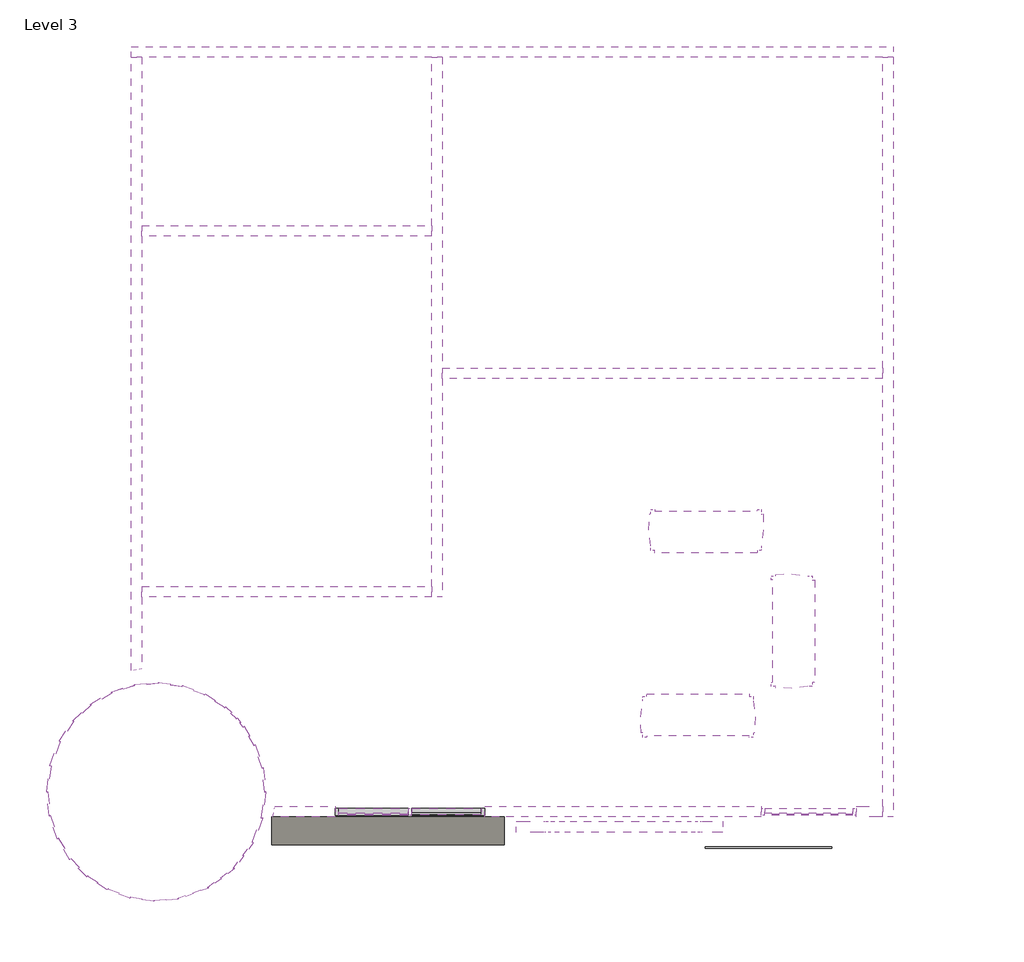
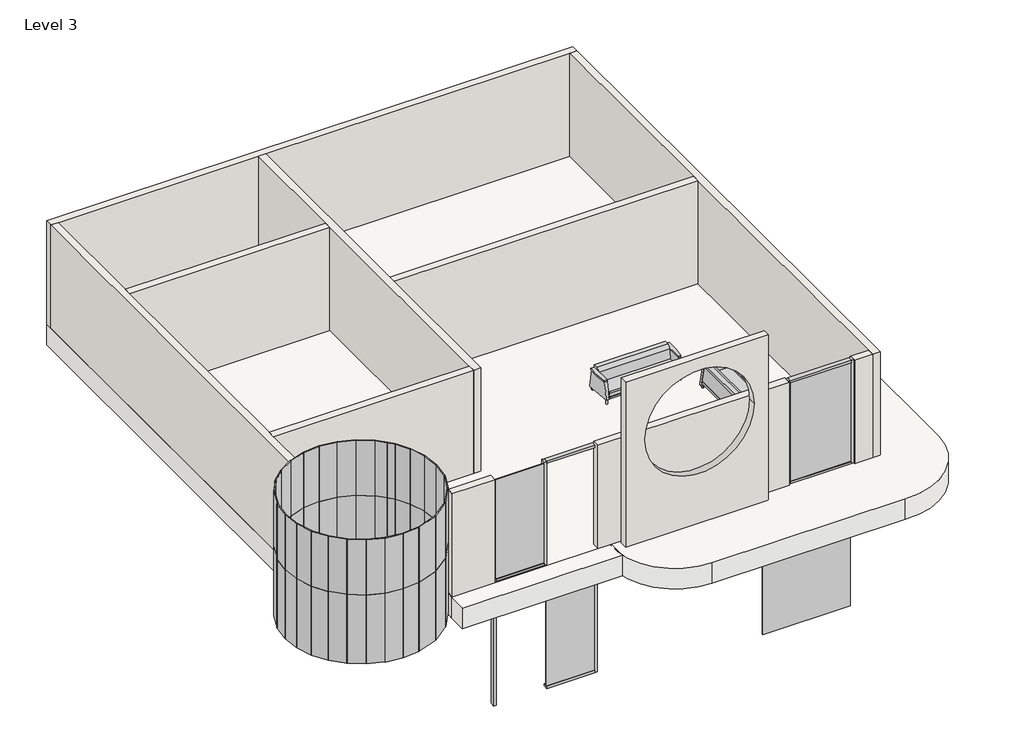
# One storey, incomplete: 60 plates, 11 members, 11 walls, 3 furniture elements, 2 slabs.
"""IFC4 building model written with IfcOpenShell, lengths in millimetres."""

from ifc_helpers import new_model, si_unit, point, frame, frame_2d, origin, place, context, project, spatial, polyline, circle_curve, trimmed, segment, composite_curve, outline, extrude, faceted_brep, transform, mapped, element, save
from ifc_brep_helpers import plane_surface, revolved_surface, advanced_brep
from components import furniture_aff9b2fb, member_eaba9652, member_3f395ae9, member_0c868e12, member_7bc42366, system_panel_glazed_f1c144f9, system_panel_glazed_8ed2b2ee, system_panel_glazed_c7815b78, system_panel_glazed_220ba5f3, system_panel_glazed_11fb153e, system_panel_glazed_2f540b85, system_panel_glazed_4848e608, system_panel_glazed_8b35a0ff, system_panel_glazed_87282c25, system_panel_glazed_6d1bb68c, system_panel_glazed_cb3ffd69, system_panel_glazed_404d015f, system_panel_glazed_7b556abe, system_panel_glazed_c60cfc80, system_panel_glazed_370bf902

model = new_model("IFC4")

# Units and contexts
model_context = context("Model", 3, world=origin())
ifc_project = project(units=[si_unit("LENGTHUNIT", "METRE", prefix="MILLI")], contexts=[model_context])

# Site, building, storey
site = spatial("IfcSite", under=ifc_project)
building = spatial("IfcBuilding", under=site)
storey = spatial("IfcBuildingStorey", under=building, Name="Level 3", Elevation=6096.0)

# Furniture
placement = place(None, origin())
furniture_shape = furniture_aff9b2fb(model_context)
element("IfcFurniture", 1, ObjectType="Sofa-Pensi : 84\"", at=placement, inside=storey, context=model_context, shape_type="MappedRepresentation", body=[
    mapped(furniture_shape, transform((-2244.8524991, 3650.1964615, 7315.2), x_axis=(1.0, 0.0, 0.0), y_axis=(0.0, 1.0, 0.0), z_axis=(0.0, 0.0, 1.0))),
])
element("IfcFurniture", 2, ObjectType="Sofa-Pensi : 84\"", at=placement, inside=storey, context=model_context, shape_type="MappedRepresentation", body=[
    mapped(furniture_shape, transform((-12.736413, 1720.492712, 7315.2), x_axis=(0.0, 1.0, 0.0), y_axis=(-1.0, 0.0, 0.0), z_axis=(0.0, 0.0, 1.0))),
])
element("IfcFurniture", 3, ObjectType="Sofa-Pensi : 84\"", at=placement, inside=storey, context=model_context, shape_type="MappedRepresentation", body=[
    mapped(furniture_shape, transform((-1840.0399991, 648.4161336, 7315.2), x_axis=(-1.0, 0.0, 0.0), y_axis=(0.0, -1.0, 0.0), z_axis=(0.0, 0.0, 1.0))),
])

# Members
member_shape = member_eaba9652(model_context)
element("IfcMember", 4, ObjectType="Rectangular Mullion : 2.5\" x 5\" rectangular", at=placement, inside=storey, context=model_context, shape_type="MappedRepresentation", body=[
    mapped(member_shape, transform((-7672.5789001, -1482.8937024, 7315.2), x_axis=(-1.0, 0.0, 0.0), y_axis=(0.0, 1.0, 0.0), z_axis=(0.0, 0.0, -1.0))),
])
member_2_shape = member_3f395ae9(model_context)
element("IfcMember", 5, ObjectType="Rectangular Mullion : 2.5\" x 5\" rectangular", at=placement, inside=storey, context=model_context, shape_type="MappedRepresentation", body=[
    mapped(member_2_shape, transform((-9111.7115512, -1482.8937024, 3657.6), x_axis=(-1.0, 0.0, 0.0), y_axis=(0.0, 1.0, 0.0), z_axis=(0.0, 0.0, -1.0))),
])
element("IfcMember", 6, ObjectType="Rectangular Mullion : 2.5\" x 5\" rectangular", at=placement, inside=storey, context=model_context, shape_type="MappedRepresentation", body=[
    mapped(member_2_shape, transform((-899.4462491, -1482.8937024, 7315.2), x_axis=(-1.0, 0.0, 0.0), y_axis=(0.0, 1.0, 0.0), z_axis=(0.0, 0.0, -1.0))),
])
element("IfcMember", 7, ObjectType="Rectangular Mullion : 2.5\" x 5\" rectangular", at=placement, inside=storey, context=model_context, shape_type="MappedRepresentation", body=[
    mapped(member_2_shape, transform((-6233.4462491, -1482.8937024, 6705.6), x_axis=(1.0, 0.0, 0.0), y_axis=(0.0, 1.0, 0.0), z_axis=(0.0, 0.0, 1.0))),
])
element("IfcMember", 8, ObjectType="Rectangular Mullion : 2.5\" x 5\" rectangular", at=placement, inside=storey, context=model_context, shape_type="MappedRepresentation", body=[
    mapped(member_2_shape, transform((929.3537509, -1482.8937024, 10363.2), x_axis=(1.0, 0.0, 0.0), y_axis=(0.0, 1.0, 0.0), z_axis=(0.0, 0.0, 1.0))),
])
member_3_shape = member_0c868e12(model_context)
element("IfcMember", 9, ObjectType="Rectangular Mullion : 2.5\" x 5\" rectangular", at=placement, inside=storey, context=model_context, shape_type="MappedRepresentation", body=[
    mapped(member_3_shape, transform((-9048.2115512, -1482.8937024, 6705.6), x_axis=(0.0, 0.0, 1.0), y_axis=(0.0, 1.0, 0.0), z_axis=(-1.0, 0.0, 0.0))),
])
element("IfcMember", 10, ObjectType="Rectangular Mullion : 2.5\" x 5\" rectangular", at=placement, inside=storey, context=model_context, shape_type="MappedRepresentation", body=[
    mapped(member_3_shape, transform((-7640.8289001, -1482.8937024, 10363.2), x_axis=(0.0, 0.0, 1.0), y_axis=(0.0, 1.0, 0.0), z_axis=(-1.0, 0.0, 0.0))),
])
element("IfcMember", 11, ObjectType="Rectangular Mullion : 2.5\" x 5\" rectangular", at=placement, inside=storey, context=model_context, shape_type="MappedRepresentation", body=[
    mapped(member_3_shape, transform((-6296.9462491, -1482.8937024, 3657.6), x_axis=(0.0, 0.0, -1.0), y_axis=(0.0, 1.0, 0.0), z_axis=(1.0, 0.0, 0.0))),
])
element("IfcMember", 12, ObjectType="Rectangular Mullion : 2.5\" x 5\" rectangular", at=placement, inside=storey, context=model_context, shape_type="MappedRepresentation", body=[
    mapped(member_3_shape, transform((-7704.3289001, -1482.8937024, 7315.2), x_axis=(0.0, 0.0, -1.0), y_axis=(0.0, 1.0, 0.0), z_axis=(1.0, 0.0, 0.0))),
])
member_4_shape = member_7bc42366(model_context)
element("IfcMember", 13, ObjectType="Rectangular Mullion : 2.5\" x 5\" rectangular", at=placement, inside=storey, context=model_context, shape_type="MappedRepresentation", body=[
    mapped(member_4_shape, transform((-835.9462491, -1482.8937024, 10363.2), x_axis=(0.0, 0.0, 1.0), y_axis=(0.0, 1.0, 0.0), z_axis=(-1.0, 0.0, 0.0))),
])
element("IfcMember", 14, ObjectType="Rectangular Mullion : 2.5\" x 5\" rectangular", at=placement, inside=storey, context=model_context, shape_type="MappedRepresentation", body=[
    mapped(member_4_shape, transform((865.8537509, -1482.8937024, 7315.2), x_axis=(0.0, 0.0, -1.0), y_axis=(0.0, 1.0, 0.0), z_axis=(1.0, 0.0, 0.0))),
])

# Plates
system_panel_glazed_shape = system_panel_glazed_f1c144f9(model_context)
element("IfcPlate", 15, ObjectType="System Panel : Glazed", at=placement, inside=storey, context=model_context, shape_type="MappedRepresentation", body=[
    mapped(system_panel_glazed_shape, transform((-14541.9245022, -346.5978939, 7315.2), x_axis=(-0.3551689475306269, -0.9348021281051873, 0.0), y_axis=(0.9348021281051873, -0.3551689475306269, 0.0), z_axis=(0.0, 0.0, 1.0))),
])
element("IfcPlate", 16, ObjectType="System Panel : Glazed", at=placement, inside=storey, context=model_context, shape_type="MappedRepresentation", body=[
    mapped(system_panel_glazed_shape, transform((-10582.1178502, -1851.0877948, 7315.2), x_axis=(0.35516894753064066, 0.934802128105182, 0.0), y_axis=(-0.934802128105182, 0.35516894753064066, 0.0), z_axis=(0.0, 0.0, 1.0))),
])
element("IfcPlate", 17, ObjectType="System Panel : Glazed", at=placement, inside=storey, context=model_context, shape_type="MappedRepresentation", body=[
    mapped(system_panel_glazed_shape, transform((-10459.5232171, -1354.5613954, 7315.2), x_axis=(0.12073632210407238, 0.9926846128175765, 0.0), y_axis=(-0.9926846128175765, 0.12073632210407238, 0.0), z_axis=(0.0, 0.0, 1.0))),
])
element("IfcPlate", 18, ObjectType="System Panel : Glazed", at=placement, inside=storey, context=model_context, shape_type="MappedRepresentation", body=[
    mapped(system_panel_glazed_shape, transform((-14664.5191354, -843.1242933, 7315.2), x_axis=(-0.12073632210406242, -0.9926846128175777, 0.0), y_axis=(0.9926846128175777, -0.12073632210406242, 0.0), z_axis=(0.0, 0.0, 1.0))),
])
system_panel_glazed_2_shape = system_panel_glazed_8ed2b2ee(model_context)
element("IfcPlate", 19, ObjectType="System Panel : Glazed", at=placement, inside=storey, context=model_context, shape_type="MappedRepresentation", body=[
    mapped(system_panel_glazed_2_shape, transform((-11841.3777431, -3082.3793017, 7315.2), x_axis=(0.9398911711666007, 0.34147413718036645, 0.0), y_axis=(-0.34147413718036645, 0.9398911711666007, 0.0), z_axis=(0.0, 0.0, 1.0))),
])
element("IfcPlate", 20, ObjectType="System Panel : Glazed", at=placement, inside=storey, context=model_context, shape_type="MappedRepresentation", body=[
    mapped(system_panel_glazed_2_shape, transform((-10858.9635423, -2345.1728692, 7315.2), x_axis=(0.5905687200141164, 0.8069873524045393, 0.0), y_axis=(-0.8069873524045393, 0.5905687200141164, 0.0), z_axis=(0.0, 0.0, 1.0))),
])
element("IfcPlate", 21, ObjectType="System Panel : Glazed", at=placement, inside=storey, context=model_context, shape_type="MappedRepresentation", body=[
    mapped(system_panel_glazed_2_shape, transform((-11295.3522982, -2786.8279712, 7315.2), x_axis=(0.7998453025525061, 0.6002062078858317, 0.0), y_axis=(-0.6002062078858317, 0.7998453025525061, 0.0), z_axis=(0.0, 0.0, 1.0))),
])
system_panel_glazed_3_shape = system_panel_glazed_c7815b78(model_context)
element("IfcPlate", 22, ObjectType="System Panel : Glazed", at=placement, inside=storey, context=model_context, shape_type="MappedRepresentation", body=[
    mapped(system_panel_glazed_3_shape, transform((-10454.4737362, -864.5204039, 7315.2), x_axis=(-0.11050163420416613, 0.993875942378227, 0.0), y_axis=(-0.993875942378227, -0.11050163420416613, 0.0), z_axis=(0.0, 0.0, 1.0))),
])
element("IfcPlate", 23, ObjectType="System Panel : Glazed", at=placement, inside=storey, context=model_context, shape_type="MappedRepresentation", body=[
    mapped(system_panel_glazed_3_shape, transform((-14669.5686163, -1333.1652848, 7315.2), x_axis=(0.11050163420415138, -0.9938759423782286, 0.0), y_axis=(0.9938759423782286, 0.11050163420415138, 0.0), z_axis=(0.0, 0.0, 1.0))),
])
element("IfcPlate", 24, ObjectType="System Panel : Glazed", at=placement, inside=storey, context=model_context, shape_type="MappedRepresentation", body=[
    mapped(system_panel_glazed_3_shape, transform((-11410.1424167, 681.5611944, 7315.2), x_axis=(-0.8396018558176894, 0.5432022861766066, 0.0), y_axis=(-0.5432022861766066, -0.8396018558176894, 0.0), z_axis=(0.0, 0.0, 1.0))),
])
element("IfcPlate", 25, ObjectType="System Panel : Glazed", at=placement, inside=storey, context=model_context, shape_type="MappedRepresentation", body=[
    mapped(system_panel_glazed_3_shape, transform((-13212.0893695, 919.590846, 7315.2), x_axis=(-0.9518517343814786, -0.3065587639506839, 0.0), y_axis=(0.3065587639506839, -0.9518517343814786, 0.0), z_axis=(0.0, 0.0, 1.0))),
])
element("IfcPlate", 26, ObjectType="System Panel : Glazed", at=placement, inside=storey, context=model_context, shape_type="MappedRepresentation", body=[
    mapped(system_panel_glazed_3_shape, transform((-12839.7224363, -3201.1142893, 7315.2), x_axis=(0.9913878918151698, -0.1309581916577702, 0.0), y_axis=(0.1309581916577702, 0.9913878918151698, 0.0), z_axis=(0.0, 0.0, 1.0))),
])
element("IfcPlate", 27, ObjectType="System Panel : Glazed", at=placement, inside=storey, context=model_context, shape_type="MappedRepresentation", body=[
    mapped(system_panel_glazed_3_shape, transform((-14365.783041, -2213.7896382, 7315.2), x_axis=(0.5257859322352114, -0.8506169252157811, 0.0), y_axis=(0.8506169252157811, 0.5257859322352114, 0.0), z_axis=(0.0, 0.0, 1.0))),
])
element("IfcPlate", 28, ObjectType="System Panel : Glazed", at=placement, inside=storey, context=model_context, shape_type="MappedRepresentation", body=[
    mapped(system_panel_glazed_3_shape, transform((-13713.8999358, -2879.2468831, 7315.2), x_axis=(0.8396018558176805, -0.5432022861766201, 0.0), y_axis=(0.5432022861766201, 0.8396018558176805, 0.0), z_axis=(0.0, 0.0, 1.0))),
])
element("IfcPlate", 29, ObjectType="System Panel : Glazed", at=placement, inside=storey, context=model_context, shape_type="MappedRepresentation", body=[
    mapped(system_panel_glazed_3_shape, transform((-14014.4059364, 446.2272921, 7315.2), x_axis=(-0.7286232370002992, -0.6849147235263715, 0.0), y_axis=(0.6849147235263715, -0.7286232370002992, 0.0), z_axis=(0.0, 0.0, 1.0))),
])
element("IfcPlate", 30, ObjectType="System Panel : Glazed", at=placement, inside=storey, context=model_context, shape_type="MappedRepresentation", body=[
    mapped(system_panel_glazed_3_shape, transform((-12284.3199161, 1003.4286006, 7315.2), x_axis=(-0.9913878918151723, 0.1309581916577514, 0.0), y_axis=(-0.1309581916577514, -0.9913878918151723, 0.0), z_axis=(0.0, 0.0, 1.0))),
])
element("IfcPlate", 31, ObjectType="System Panel : Glazed", at=placement, inside=storey, context=model_context, shape_type="MappedRepresentation", body=[
    mapped(system_panel_glazed_3_shape, transform((-12752.8652893, 1013.0855973, 7315.2), x_axis=(-0.9959419324521102, -0.08999815100076568, 0.0), y_axis=(0.08999815100076568, -0.9959419324521102, 0.0), z_axis=(0.0, 0.0, 1.0))),
])
element("IfcPlate", 32, ObjectType="System Panel : Glazed", at=placement, inside=storey, context=model_context, shape_type="MappedRepresentation", body=[
    mapped(system_panel_glazed_3_shape, transform((-11829.3381514, 891.0915272, 7315.2), x_axis=(-0.9384120429483949, 0.34551821608913763, 0.0), y_axis=(-0.34551821608913763, -0.9384120429483949, 0.0), z_axis=(0.0, 0.0, 1.0))),
])
element("IfcPlate", 33, ObjectType="System Panel : Glazed", at=placement, inside=storey, context=model_context, shape_type="MappedRepresentation", body=[
    mapped(system_panel_glazed_3_shape, transform((-10557.4115054, -407.3204039, 7315.2), x_axis=(-0.3261077326604367, 0.9453326116764772, 0.0), y_axis=(-0.9453326116764772, -0.3261077326604367, 0.0), z_axis=(0.0, 0.0, 1.0))),
])
element("IfcPlate", 34, ObjectType="System Panel : Glazed", at=placement, inside=storey, context=model_context, shape_type="MappedRepresentation", body=[
    mapped(system_panel_glazed_3_shape, transform((-12371.1770631, -3210.771286, 7315.2), x_axis=(0.9959419324521115, 0.08999815100075, 0.0), y_axis=(-0.08999815100075, 0.9959419324521115, 0.0), z_axis=(0.0, 0.0, 1.0))),
])
element("IfcPlate", 35, ObjectType="System Panel : Glazed", at=placement, inside=storey, context=model_context, shape_type="MappedRepresentation", body=[
    mapped(system_panel_glazed_3_shape, transform((-13294.7042011, -3088.7772159, 7315.2), x_axis=(0.9384120429483891, -0.34551821608915334, 0.0), y_axis=(0.34551821608915334, 0.9384120429483891, 0.0), z_axis=(0.0, 0.0, 1.0))),
])
element("IfcPlate", 36, ObjectType="System Panel : Glazed", at=placement, inside=storey, context=model_context, shape_type="MappedRepresentation", body=[
    mapped(system_panel_glazed_3_shape, transform((-14076.8350959, -2582.7572647, 7315.2), x_axis=(0.6997834615185511, -0.7143550286692988, 0.0), y_axis=(0.7143550286692988, 0.6997834615185511, 0.0), z_axis=(0.0, 0.0, 1.0))),
])
element("IfcPlate", 37, ObjectType="System Panel : Glazed", at=placement, inside=storey, context=model_context, shape_type="MappedRepresentation", body=[
    mapped(system_panel_glazed_3_shape, transform((-14566.6308471, -1790.3652848, 7315.2), x_axis=(0.32610773266042153, -0.9453326116764824, 0.0), y_axis=(0.9453326116764824, 0.32610773266042153, 0.0), z_axis=(0.0, 0.0, 1.0))),
])
element("IfcPlate", 38, ObjectType="System Panel : Glazed", at=placement, inside=storey, context=model_context, shape_type="MappedRepresentation", body=[
    mapped(system_panel_glazed_3_shape, transform((-14318.3113206, 89.4787227, 7315.2), x_axis=(-0.5603879632167612, -0.8282302401396425, 0.0), y_axis=(0.8282302401396425, -0.5603879632167612, 0.0), z_axis=(0.0, 0.0, 1.0))),
])
element("IfcPlate", 39, ObjectType="System Panel : Glazed", at=placement, inside=storey, context=model_context, shape_type="MappedRepresentation", body=[
    mapped(system_panel_glazed_3_shape, transform((-13639.5625299, 727.5108588, 7315.2), x_axis=(-0.8612707706620223, -0.508146297441245, 0.0), y_axis=(0.508146297441245, -0.8612707706620223, 0.0), z_axis=(0.0, 0.0, 1.0))),
])
system_panel_glazed_4_shape = system_panel_glazed_220ba5f3(model_context)
element("IfcPlate", 40, ObjectType="System Panel : Glazed", at=placement, inside=storey, context=model_context, shape_type="MappedRepresentation", body=[
    mapped(system_panel_glazed_4_shape, transform((-10742.3305673, -4.7597883, 7315.2), x_axis=(-0.5152811917631037, 0.8570211744263939, 0.0), y_axis=(-0.8570211744263939, -0.5152811917631037, 0.0), z_axis=(0.0, 0.0, 1.0))),
])
system_panel_glazed_5_shape = system_panel_glazed_11fb153e(model_context)
element("IfcPlate", 41, ObjectType="System Panel : Glazed", at=placement, inside=storey, context=model_context, shape_type="MappedRepresentation", body=[
    mapped(system_panel_glazed_5_shape, transform((-11098.0043985, 445.2241463, 7315.2), x_axis=(-0.7256671855033587, 0.6880458821064435, 0.0), y_axis=(-0.6880458821064435, -0.7256671855033587, 0.0), z_axis=(0.0, 0.0, 1.0))),
])
system_panel_glazed_6_shape = system_panel_glazed_2f540b85(model_context)
element("IfcPlate", 42, ObjectType="System Panel : Glazed", at=placement, inside=storey, context=model_context, shape_type="MappedRepresentation", body=[
    mapped(system_panel_glazed_6_shape, transform((-10917.0903061, 255.9395759, 7315.2), x_axis=(-0.6357445726375757, 0.7718995001694627, 0.0), y_axis=(-0.7718995001694627, -0.6357445726375757, 0.0), z_axis=(0.0, 0.0, 1.0))),
])
system_panel_glazed_7_shape = system_panel_glazed_4848e608(model_context)
element("IfcPlate", 43, ObjectType="System Panel : Glazed", at=placement, inside=storey, context=model_context, shape_type="MappedRepresentation", body=[
    mapped(system_panel_glazed_7_shape, transform((-14669.5686163, -1333.1652848, 9347.2), x_axis=(0.11050163420415138, -0.9938759423782286, 0.0), y_axis=(0.9938759423782286, 0.11050163420415138, 0.0), z_axis=(0.0, 0.0, 1.0))),
])
element("IfcPlate", 44, ObjectType="System Panel : Glazed", at=placement, inside=storey, context=model_context, shape_type="MappedRepresentation", body=[
    mapped(system_panel_glazed_7_shape, transform((-14365.783041, -2213.7896382, 9347.2), x_axis=(0.5257859322352114, -0.8506169252157811, 0.0), y_axis=(0.8506169252157811, 0.5257859322352114, 0.0), z_axis=(0.0, 0.0, 1.0))),
])
element("IfcPlate", 45, ObjectType="System Panel : Glazed", at=placement, inside=storey, context=model_context, shape_type="MappedRepresentation", body=[
    mapped(system_panel_glazed_7_shape, transform((-13713.8999358, -2879.2468831, 9347.2), x_axis=(0.8396018558176805, -0.5432022861766201, 0.0), y_axis=(0.5432022861766201, 0.8396018558176805, 0.0), z_axis=(0.0, 0.0, 1.0))),
])
element("IfcPlate", 46, ObjectType="System Panel : Glazed", at=placement, inside=storey, context=model_context, shape_type="MappedRepresentation", body=[
    mapped(system_panel_glazed_7_shape, transform((-12839.7224363, -3201.1142893, 9347.2), x_axis=(0.9913878918151698, -0.13095819165777017, 0.0), y_axis=(0.13095819165777017, 0.9913878918151698, 0.0), z_axis=(0.0, 0.0, 1.0))),
])
element("IfcPlate", 47, ObjectType="System Panel : Glazed", at=placement, inside=storey, context=model_context, shape_type="MappedRepresentation", body=[
    mapped(system_panel_glazed_7_shape, transform((-12371.1770631, -3210.771286, 9347.2), x_axis=(0.9959419324521115, 0.08999815100075002, 0.0), y_axis=(-0.08999815100075002, 0.9959419324521115, 0.0), z_axis=(0.0, 0.0, 1.0))),
])
element("IfcPlate", 48, ObjectType="System Panel : Glazed", at=placement, inside=storey, context=model_context, shape_type="MappedRepresentation", body=[
    mapped(system_panel_glazed_7_shape, transform((-13294.7042011, -3088.7772159, 9347.2), x_axis=(0.9384120429483891, -0.34551821608915334, 0.0), y_axis=(0.34551821608915334, 0.9384120429483891, 0.0), z_axis=(0.0, 0.0, 1.0))),
])
element("IfcPlate", 49, ObjectType="System Panel : Glazed", at=placement, inside=storey, context=model_context, shape_type="MappedRepresentation", body=[
    mapped(system_panel_glazed_7_shape, transform((-14076.8350959, -2582.7572647, 9347.2), x_axis=(0.6997834615185511, -0.7143550286692988, 0.0), y_axis=(0.7143550286692988, 0.6997834615185511, 0.0), z_axis=(0.0, 0.0, 1.0))),
])
element("IfcPlate", 50, ObjectType="System Panel : Glazed", at=placement, inside=storey, context=model_context, shape_type="MappedRepresentation", body=[
    mapped(system_panel_glazed_7_shape, transform((-14566.6308471, -1790.3652848, 9347.2), x_axis=(0.32610773266042153, -0.9453326116764824, 0.0), y_axis=(0.9453326116764824, 0.32610773266042153, 0.0), z_axis=(0.0, 0.0, 1.0))),
])
element("IfcPlate", 51, ObjectType="System Panel : Glazed", at=placement, inside=storey, context=model_context, shape_type="MappedRepresentation", body=[
    mapped(system_panel_glazed_7_shape, transform((-10454.4737362, -864.5204039, 9347.2), x_axis=(-0.11050163420416614, 0.993875942378227, 0.0), y_axis=(-0.993875942378227, -0.11050163420416614, 0.0), z_axis=(0.0, 0.0, 1.0))),
])
element("IfcPlate", 52, ObjectType="System Panel : Glazed", at=placement, inside=storey, context=model_context, shape_type="MappedRepresentation", body=[
    mapped(system_panel_glazed_7_shape, transform((-10557.4115054, -407.3204039, 9347.2), x_axis=(-0.32610773266043674, 0.9453326116764772, 0.0), y_axis=(-0.9453326116764772, -0.32610773266043674, 0.0), z_axis=(0.0, 0.0, 1.0))),
])
element("IfcPlate", 53, ObjectType="System Panel : Glazed", at=placement, inside=storey, context=model_context, shape_type="MappedRepresentation", body=[
    mapped(system_panel_glazed_7_shape, transform((-11410.1424167, 681.5611944, 9347.2), x_axis=(-0.8396018558176894, 0.5432022861766066, 0.0), y_axis=(-0.5432022861766066, -0.8396018558176894, 0.0), z_axis=(0.0, 0.0, 1.0))),
])
element("IfcPlate", 54, ObjectType="System Panel : Glazed", at=placement, inside=storey, context=model_context, shape_type="MappedRepresentation", body=[
    mapped(system_panel_glazed_7_shape, transform((-11829.3381514, 891.0915272, 9347.2), x_axis=(-0.9384120429483949, 0.34551821608913763, 0.0), y_axis=(-0.34551821608913763, -0.9384120429483949, 0.0), z_axis=(0.0, 0.0, 1.0))),
])
element("IfcPlate", 55, ObjectType="System Panel : Glazed", at=placement, inside=storey, context=model_context, shape_type="MappedRepresentation", body=[
    mapped(system_panel_glazed_7_shape, transform((-12284.3199161, 1003.4286006, 9347.2), x_axis=(-0.9913878918151723, 0.13095819165775144, 0.0), y_axis=(-0.13095819165775144, -0.9913878918151723, 0.0), z_axis=(0.0, 0.0, 1.0))),
])
element("IfcPlate", 56, ObjectType="System Panel : Glazed", at=placement, inside=storey, context=model_context, shape_type="MappedRepresentation", body=[
    mapped(system_panel_glazed_7_shape, transform((-12752.8652893, 1013.0855973, 9347.2), x_axis=(-0.9959419324521102, -0.08999815100076569, 0.0), y_axis=(0.08999815100076569, -0.9959419324521102, 0.0), z_axis=(0.0, 0.0, 1.0))),
])
element("IfcPlate", 57, ObjectType="System Panel : Glazed", at=placement, inside=storey, context=model_context, shape_type="MappedRepresentation", body=[
    mapped(system_panel_glazed_7_shape, transform((-13212.0893695, 919.590846, 9347.2), x_axis=(-0.9518517343814786, -0.3065587639506839, 0.0), y_axis=(0.3065587639506839, -0.9518517343814786, 0.0), z_axis=(0.0, 0.0, 1.0))),
])
element("IfcPlate", 58, ObjectType="System Panel : Glazed", at=placement, inside=storey, context=model_context, shape_type="MappedRepresentation", body=[
    mapped(system_panel_glazed_7_shape, transform((-13639.5625299, 727.5108588, 9347.2), x_axis=(-0.8612707706620224, -0.5081462974412448, 0.0), y_axis=(0.5081462974412448, -0.8612707706620224, 0.0), z_axis=(0.0, 0.0, 1.0))),
])
element("IfcPlate", 59, ObjectType="System Panel : Glazed", at=placement, inside=storey, context=model_context, shape_type="MappedRepresentation", body=[
    mapped(system_panel_glazed_7_shape, transform((-14014.4059364, 446.2272921, 9347.2), x_axis=(-0.7286232370002992, -0.6849147235263715, 0.0), y_axis=(0.6849147235263715, -0.7286232370002992, 0.0), z_axis=(0.0, 0.0, 1.0))),
])
element("IfcPlate", 60, ObjectType="System Panel : Glazed", at=placement, inside=storey, context=model_context, shape_type="MappedRepresentation", body=[
    mapped(system_panel_glazed_7_shape, transform((-14318.3113206, 89.4787227, 9347.2), x_axis=(-0.5603879632167612, -0.8282302401396425, 0.0), y_axis=(0.8282302401396425, -0.5603879632167612, 0.0), z_axis=(0.0, 0.0, 1.0))),
])
system_panel_glazed_8_shape = system_panel_glazed_8b35a0ff(model_context)
element("IfcPlate", 61, ObjectType="System Panel : Glazed", at=placement, inside=storey, context=model_context, shape_type="MappedRepresentation", body=[
    mapped(system_panel_glazed_8_shape, transform((-10742.3305673, -4.7597883, 9347.2), x_axis=(-0.5152811917631037, 0.8570211744263939, 0.0), y_axis=(-0.8570211744263939, -0.5152811917631037, 0.0), z_axis=(0.0, 0.0, 1.0))),
])
system_panel_glazed_9_shape = system_panel_glazed_87282c25(model_context)
element("IfcPlate", 62, ObjectType="System Panel : Glazed", at=placement, inside=storey, context=model_context, shape_type="MappedRepresentation", body=[
    mapped(system_panel_glazed_9_shape, transform((-10917.0903061, 255.9395759, 9347.2), x_axis=(-0.6357445726375757, 0.7718995001694627, 0.0), y_axis=(-0.7718995001694627, -0.6357445726375757, 0.0), z_axis=(0.0, 0.0, 1.0))),
])
system_panel_glazed_10_shape = system_panel_glazed_6d1bb68c(model_context)
element("IfcPlate", 63, ObjectType="System Panel : Glazed", at=placement, inside=storey, context=model_context, shape_type="MappedRepresentation", body=[
    mapped(system_panel_glazed_10_shape, transform((-11098.0043985, 445.2241463, 9347.2), x_axis=(-0.7256671855033587, 0.6880458821064435, 0.0), y_axis=(-0.6880458821064435, -0.7256671855033587, 0.0), z_axis=(0.0, 0.0, 1.0))),
])
system_panel_glazed_11_shape = system_panel_glazed_cb3ffd69(model_context)
element("IfcPlate", 64, ObjectType="System Panel : Glazed", at=placement, inside=storey, context=model_context, shape_type="MappedRepresentation", body=[
    mapped(system_panel_glazed_11_shape, transform((-10582.1178502, -1851.0877948, 9347.2), x_axis=(0.3551689475306406, 0.934802128105182, 0.0), y_axis=(-0.934802128105182, 0.3551689475306406, 0.0), z_axis=(0.0, 0.0, 1.0))),
])
element("IfcPlate", 65, ObjectType="System Panel : Glazed", at=placement, inside=storey, context=model_context, shape_type="MappedRepresentation", body=[
    mapped(system_panel_glazed_11_shape, transform((-10459.5232171, -1354.5613954, 9347.2), x_axis=(0.12073632210407237, 0.9926846128175765, 0.0), y_axis=(-0.9926846128175765, 0.12073632210407237, 0.0), z_axis=(0.0, 0.0, 1.0))),
])
element("IfcPlate", 66, ObjectType="System Panel : Glazed", at=placement, inside=storey, context=model_context, shape_type="MappedRepresentation", body=[
    mapped(system_panel_glazed_11_shape, transform((-14541.9245022, -346.5978939, 9347.2), x_axis=(-0.35516894753062683, -0.9348021281051873, 0.0), y_axis=(0.9348021281051873, -0.35516894753062683, 0.0), z_axis=(0.0, 0.0, 1.0))),
])
element("IfcPlate", 67, ObjectType="System Panel : Glazed", at=placement, inside=storey, context=model_context, shape_type="MappedRepresentation", body=[
    mapped(system_panel_glazed_11_shape, transform((-14664.5191354, -843.1242933, 9347.2), x_axis=(-0.12073632210406242, -0.9926846128175777, 0.0), y_axis=(0.9926846128175777, -0.12073632210406242, 0.0), z_axis=(0.0, 0.0, 1.0))),
])
system_panel_glazed_12_shape = system_panel_glazed_404d015f(model_context)
element("IfcPlate", 68, ObjectType="System Panel : Glazed", at=placement, inside=storey, context=model_context, shape_type="MappedRepresentation", body=[
    mapped(system_panel_glazed_12_shape, transform((-11841.3777431, -3082.3793017, 9347.2), x_axis=(0.9398911711666007, 0.34147413718036645, 0.0), y_axis=(-0.34147413718036645, 0.9398911711666007, 0.0), z_axis=(0.0, 0.0, 1.0))),
])
element("IfcPlate", 69, ObjectType="System Panel : Glazed", at=placement, inside=storey, context=model_context, shape_type="MappedRepresentation", body=[
    mapped(system_panel_glazed_12_shape, transform((-10858.9635423, -2345.1728692, 9347.2), x_axis=(0.5905687200141164, 0.8069873524045393, 0.0), y_axis=(-0.8069873524045393, 0.5905687200141164, 0.0), z_axis=(0.0, 0.0, 1.0))),
])
element("IfcPlate", 70, ObjectType="System Panel : Glazed", at=placement, inside=storey, context=model_context, shape_type="MappedRepresentation", body=[
    mapped(system_panel_glazed_12_shape, transform((-11295.3522982, -2786.8279712, 9347.2), x_axis=(0.7998453025525061, 0.6002062078858317, 0.0), y_axis=(-0.6002062078858317, 0.7998453025525061, 0.0), z_axis=(0.0, 0.0, 1.0))),
])
system_panel_glazed_13_shape = system_panel_glazed_7b556abe(model_context)
element("IfcPlate", 71, ObjectType="System Panel : Glazed", at=placement, inside=storey, context=model_context, shape_type="MappedRepresentation", body=[
    mapped(system_panel_glazed_13_shape, transform((-6968.8875746, -1482.8937024, 3721.1), x_axis=(-1.0, 0.0, 0.0), y_axis=(0.0, -1.0, 0.0), z_axis=(0.0, 0.0, 1.0))),
])
element("IfcPlate", 72, ObjectType="System Panel : Glazed", at=placement, inside=storey, context=model_context, shape_type="MappedRepresentation", body=[
    mapped(system_panel_glazed_13_shape, transform((-8376.2702257, -1482.8937024, 7378.7), x_axis=(-1.0, 0.0, 0.0), y_axis=(0.0, -1.0, 0.0), z_axis=(0.0, 0.0, 1.0))),
])
system_panel_glazed_14_shape = system_panel_glazed_c60cfc80(model_context)
element("IfcPlate", 73, ObjectType="System Panel : Glazed", at=placement, inside=storey, context=model_context, shape_type="MappedRepresentation", body=[
    mapped(system_panel_glazed_14_shape, transform((-759.7462491, -2143.2937024, 3657.6), x_axis=(-1.0, 0.0, 0.0), y_axis=(0.0, -1.0, 0.0), z_axis=(0.0, 0.0, 1.0))),
])
system_panel_glazed_15_shape = system_panel_glazed_370bf902(model_context)
element("IfcPlate", 74, ObjectType="System Panel : Glazed", at=placement, inside=storey, context=model_context, shape_type="MappedRepresentation", body=[
    mapped(system_panel_glazed_15_shape, transform((14.9537509, -1482.8937024, 7378.7), x_axis=(-1.0, 0.0, 0.0), y_axis=(0.0, -1.0, 0.0), z_axis=(0.0, 0.0, 1.0))),
])

# Slabs
element("IfcSlab", 75, ObjectType="Generic - 2'", at=placement, inside=storey, context=model_context, shape_type="SweptSolid", body=[
    extrude(outline(composite_curve([segment(polyline([(3266.1537509, 13274.5062976), (3266.1537509, -1051.0937024), (3266.1537509, -1584.4937024)]), True, "CONTINUOUS"), segment(trimmed(circle_curve(frame_2d((1372.339577, -1584.4937024)), 1893.8141739), [point((3266.1537509, -1584.4937024))], [point((1259.5537509, -3474.9464215))], False, "CARTESIAN"), True, "CONTINUOUS"), segment(polyline([(1259.5537509, -3474.9464215), (-4150.6462491, -3474.9464215)]), True, "CONTINUOUS"), segment(trimmed(circle_curve(frame_2d((-4150.6462491, -1726.5731554)), 1748.373266), [point((-4150.6462491, -3474.9464215))], [point((-5893.2366015, -1584.4888812))], False, "CARTESIAN"), True, "CONTINUOUS"), segment(polyline([(-5893.2366015, -1584.4888812), (-10332.0092804, -1584.4888812)]), True, "CONTINUOUS"), segment(trimmed(circle_curve(frame_2d((-12603.9144952, -1051.2259771)), 2333.6500658), [point((-10332.0092804, -1584.4888812))], [point((-13040.6462491, 1241.1937063))], True, "CARTESIAN"), True, "CONTINUOUS"), segment(polyline([(-13040.6462491, 1241.1937063), (-13040.6462491, 13274.5062976), (3266.1537509, 13274.5062976)]), True, "CONTINUOUS")], self_intersect=False)), frame((0.0, 0.0, 6705.6), z_axis=(0.0, 0.0, 1.0), x_axis=(1.0, 0.0, 0.0)), (0.0, 0.0, 1.0), 609.6),
])
element("IfcSlab", 76, ObjectType="Generic - 2'", at=placement, inside=storey, context=model_context, shape_type="SweptSolid", body=[
    extrude(outline(polyline([(-5854.6642381, -1584.4888812), (-5854.6642381, -2117.8937024), (-10332.0092804, -2117.8937024), (-10332.0092804, -1584.4888812), (-5854.6642381, -1584.4888812)])), frame((0.0, 0.0, 6705.6), z_axis=(0.0, 0.0, 1.0), x_axis=(1.0, 0.0, 0.0)), (0.0, 0.0, 1.0), 609.6),
])

# Walls
element("IfcWall", 77, ObjectType="Generic - 8\"", at=placement, inside=storey, context=model_context, shape_type="Brep", body=[
    faceted_brep([(-13040.6462491, 13071.3062976, 7315.2), (-12837.4462491, 13071.3062976, 7315.2), (-7249.4462491, 13071.3062976, 7315.2), (-7046.2462491, 13071.3062976, 7315.2), (1437.3537509, 13071.3062976, 7315.2), (1640.5537509, 13071.3062976, 7315.2), (1640.5537509, 13071.3062976, 10363.2), (1437.3537509, 13071.3062976, 10363.2), (-7046.2462491, 13071.3062976, 10363.2), (-7249.4462491, 13071.3062976, 10363.2), (-12837.4462491, 13071.3062976, 10363.2), (-13040.6462491, 13071.3062976, 10363.2), (-13040.6462491, 13274.5062976, 7315.2), (-13040.6462491, 13274.5062976, 10363.2), (1640.5537509, 13274.5062976, 10363.2), (1640.5537509, 13274.5062976, 7315.2)], [[[0, 1, 2, 3, 4, 5, 6, 7, 8, 9, 10, 11]], [[12, 13, 14, 15]], [[5, 4, 3, 2, 1, 0, 12, 15]], [[11, 10, 9, 8, 7, 6, 14, 13]], [[6, 5, 15, 14]], [[0, 11, 13, 12]]]),
])
element("IfcWall", 78, ObjectType="Generic - 8\"", at=placement, inside=storey, context=model_context, shape_type="Brep", body=[
    faceted_brep([(1437.3537509, 13071.3062976, 7315.2), (1437.3537509, 7076.9062976, 7315.2), (1437.3537509, 6873.7062976, 7315.2), (1437.3537509, -1381.2937024, 7315.2), (1437.3537509, -1584.4937024, 7315.2), (1437.3537509, -1584.4937024, 10363.2), (1437.3537509, -1381.2937024, 10363.2), (1437.3537509, 6873.7062976, 10363.2), (1437.3537509, 7076.9062976, 10363.2), (1437.3537509, 13071.3062976, 10363.2), (1640.5537509, 13071.3062976, 7315.2), (1640.5537509, 13071.3062976, 10363.2), (1640.5537509, -1584.4937024, 10363.2), (1640.5537509, -1584.4937024, 7315.2)], [[[0, 1, 2, 3, 4, 5, 6, 7, 8, 9]], [[10, 11, 12, 13]], [[4, 3, 2, 1, 0, 10, 13]], [[9, 8, 7, 6, 5, 12, 11]], [[0, 9, 11, 10]], [[5, 4, 13, 12]]]),
])
element("IfcWall", 79, ObjectType="Generic - 8\"", at=placement, inside=storey, context=model_context, shape_type="AdvancedBrep", body=[
    advanced_brep(
    [(-13040.6462491, 13071.3062976, 7315.2), (-13040.6462491, 1241.1937063, 7315.2), (-13040.6462491, 1241.1937063, 10363.2), (-13040.6462491, 13071.3062976, 10363.2), (-12837.4462491, 13071.3062976, 7315.2), (-12837.4462491, 13071.3062976, 10363.2), (-12837.4462491, 9820.1062976, 10363.2), (-12837.4462491, 9616.9062976, 10363.2), (-12837.4462491, 2862.698962, 10363.2), (-12837.4462491, 2659.498962, 10363.2), (-12837.4462491, 1269.6553935, 10363.2), (-12837.4462491, 1269.6553935, 7315.2), (-12837.4462491, 2659.498962, 7315.2), (-12837.4462491, 2862.698962, 7315.2), (-12837.4462491, 9616.9062976, 7315.2), (-12837.4462491, 9820.1062976, 7315.2)],
    [
        (0, 1),
        (1, 2),
        (2, 3),
        (3, 0),
        (4, 5),
        (5, 6),
        (6, 7),
        (7, 8),
        (8, 9),
        (9, 10),
        (10, 11),
        (11, 12),
        (12, 13),
        (13, 14),
        (14, 15),
        (15, 4),
        (0, 4),
        (11, 1, circle_curve(frame((-12612.6150686, -1075.1054509, 7315.2), z_axis=(0.0, 0.0, 1.0), x_axis=(1.0, 0.0, 0.0)), 2355.5153315)),
        (2, 10, circle_curve(frame((-12612.6150686, -1075.1054509, 10363.2), z_axis=(0.0, 0.0, -1.0), x_axis=(1.0, 0.0, 0.0)), 2355.5153315)),
        (5, 3),
    ],
    [
        plane_surface(frame((-13040.6462491, 16068.5062976, 7315.2), z_axis=(-1.0, 0.0, 0.0), x_axis=(0.0, -1.0, 0.0))),
        plane_surface(frame((-12837.4462491, 16068.5062976, 7315.2), z_axis=(1.0, 0.0, 0.0), x_axis=(0.0, 1.0, 0.0))),
        plane_surface(frame((-13040.6462491, 13172.9062976, 7315.2), z_axis=(0.0, 0.0, -1.0), x_axis=(1.0, 0.0, 0.0))),
        plane_surface(frame((-13040.6462491, 1155.046339, 10363.2), z_axis=(0.0, 0.0, 1.0), x_axis=(1.0, 0.0, 0.0))),
        plane_surface(frame((-16139.4462491, 13071.3062976, 7315.2), z_axis=(0.0, 1.0, 0.0), x_axis=(1.0, 0.0, 0.0))),
        revolved_surface(polyline([(-10257.099737100001, -1075.1054509, 10363.2), (-10257.099737100001, -1075.1054509, 7315.2)]), (-12612.6150686, -1075.1054509, 7315.2), (0.0, 0.0, 1.0)),
    ],
    [
        (0, [[1, 2, 3, 4]]),
        (1, [[5, 6, 7, 8, 9, 10, 11, 12, 13, 14, 15, 16]]),
        (2, [[-1, 17, -16, -15, -14, -13, -12, 18]]),
        (3, [[-3, 19, -10, -9, -8, -7, -6, 20]]),
        (4, [[-4, -20, -5, -17]]),
        (5, [[-2, -18, -11, -19]]),
    ],
),
])
element("IfcWall", 80, ObjectType="Generic - 8\"", at=placement, inside=storey, context=model_context, shape_type="Brep", body=[
    faceted_brep([(-7249.4462491, 13071.3062976, 7315.2), (-7249.4462491, 9820.1062976, 7315.2), (-7249.4462491, 9616.9062976, 7315.2), (-7249.4462491, 2862.698962, 7315.2), (-7249.4462491, 2659.498962, 7315.2), (-7249.4462491, 2659.498962, 10363.2), (-7249.4462491, 2862.698962, 10363.2), (-7249.4462491, 9616.9062976, 10363.2), (-7249.4462491, 9820.1062976, 10363.2), (-7249.4462491, 13071.3062976, 10363.2), (-7046.2462491, 13071.3062976, 7315.2), (-7046.2462491, 13071.3062976, 10363.2), (-7046.2462491, 7076.9062976, 10363.2), (-7046.2462491, 6873.7062976, 10363.2), (-7046.2462491, 2659.498962, 10363.2), (-7046.2462491, 2659.498962, 7315.2), (-7046.2462491, 6873.7062976, 7315.2), (-7046.2462491, 7076.9062976, 7315.2)], [[[0, 1, 2, 3, 4, 5, 6, 7, 8, 9]], [[10, 11, 12, 13, 14, 15, 16, 17]], [[4, 3, 2, 1, 0, 10, 17, 16, 15]], [[9, 8, 7, 6, 5, 14, 13, 12, 11]], [[0, 9, 11, 10]], [[5, 4, 15, 14]]]),
])
element("IfcWall", 81, ObjectType="Generic - 8\"", at=placement, inside=storey, context=model_context, shape_type="SweptSolid", body=[
    extrude(outline(polyline([(1437.3537509, 6873.7062976), (-7046.2462491, 6873.7062976), (-7046.2462491, 7076.9062976), (1437.3537509, 7076.9062976), (1437.3537509, 6873.7062976)])), frame((0.0, 0.0, 7315.2), z_axis=(0.0, 0.0, 1.0), x_axis=(1.0, 0.0, 0.0)), (0.0, 0.0, 1.0), 3048.0),
])
element("IfcWall", 82, ObjectType="Generic - 8\"", at=placement, inside=storey, context=model_context, shape_type="SweptSolid", body=[
    extrude(outline(polyline([(-12837.4462491, 9820.1062976), (-7249.4462491, 9820.1062976), (-7249.4462491, 9616.9062976), (-12837.4462491, 9616.9062976), (-12837.4462491, 9820.1062976)])), frame((0.0, 0.0, 7315.2), z_axis=(0.0, 0.0, 1.0), x_axis=(1.0, 0.0, 0.0)), (0.0, 0.0, 1.0), 3048.0),
])
element("IfcWall", 83, ObjectType="Generic - 8\"", at=placement, inside=storey, context=model_context, shape_type="SweptSolid", body=[
    extrude(outline(polyline([(-12837.4462491, 2862.698962), (-7249.4462491, 2862.698962), (-7249.4462491, 2659.498962), (-12837.4462491, 2659.498962), (-12837.4462491, 2862.698962)])), frame((0.0, 0.0, 7315.2), z_axis=(0.0, 0.0, 1.0), x_axis=(1.0, 0.0, 0.0)), (0.0, 0.0, 1.0), 3048.0),
])
element("IfcWall", 84, ObjectType="Generic - 8\"", at=placement, inside=storey, context=model_context, shape_type="SweptSolid", body=[
    extrude(outline(composite_curve([segment(polyline([(-9111.7115512, -1584.4937024), (-10312.8376694, -1584.4937024)]), True, "CONTINUOUS"), segment(trimmed(circle_curve(frame_2d((-12612.6150686, -1075.1054509)), 2355.5153315), [point((-10312.8376694, -1584.4937024))], [point((-10277.0848865, -1381.2937024))], True, "CARTESIAN"), True, "CONTINUOUS"), segment(polyline([(-10277.0848865, -1381.2937024), (-9111.7115512, -1381.2937024), (-9111.7115512, -1584.4937024)]), True, "CONTINUOUS")], self_intersect=False)), frame((0.0, 0.0, 7315.2), z_axis=(0.0, 0.0, 1.0), x_axis=(1.0, 0.0, 0.0)), (0.0, 0.0, 1.0), 3048.0),
])
element("IfcWall", 85, ObjectType="Generic - 8\"", at=placement, inside=storey, context=model_context, shape_type="SweptSolid", body=[
    extrude(outline(polyline([(-899.4462491, -1584.4937024), (-6233.4462491, -1584.4937024), (-6233.4462491, -1381.2937024), (-899.4462491, -1381.2937024), (-899.4462491, -1584.4937024)])), frame((0.0, 0.0, 7315.2), z_axis=(0.0, 0.0, 1.0), x_axis=(1.0, 0.0, 0.0)), (0.0, 0.0, 1.0), 3048.0),
])
element("IfcWall", 86, ObjectType="Generic - 8\"", at=placement, inside=storey, context=model_context, shape_type="SweptSolid", body=[
    extrude(outline(polyline([(929.3537509, -1381.2937024), (1437.3537509, -1381.2937024), (1437.3537509, -1584.4937024), (929.3537509, -1584.4937024), (929.3537509, -1381.2937024)])), frame((0.0, 0.0, 7315.2), z_axis=(0.0, 0.0, 1.0), x_axis=(1.0, 0.0, 0.0)), (0.0, 0.0, 1.0), 3048.0),
])
element("IfcWall", 87, ObjectType="Generic - 8\"", at=placement, inside=storey, context=model_context, shape_type="SweptSolid", body=[
    extrude(outline(polyline([(7315.2, -5626.1321313), (7315.2, -1645.1788554), (12192.0, -1645.1788554), (12192.0, -5626.1321313), (7315.2, -5626.1321313)]), holes=[composite_curve([segment(trimmed(circle_curve(frame_2d((10304.1405965, -3565.033193)), 1524.0), [point((10304.1405965, -2041.033193))], [point((10304.1405965, -5089.033193))], True, "CARTESIAN"), True, "CONTINUOUS"), segment(trimmed(circle_curve(frame_2d((10304.1405965, -3565.033193)), 1524.0), [point((10304.1405965, -5089.033193))], [point((10304.1405965, -2041.033193))], True, "CARTESIAN"), True, "CONTINUOUS")], self_intersect=False)]), frame((0.0, -1873.8964354, 0.0), z_axis=(0.0, 1.0, 0.0), x_axis=(0.0, 0.0, 1.0)), (0.0, 0.0, 1.0), 203.2),
])

save(model, "model.ifc")

# Revit data of these elements
# Type "Sofa-Pensi : 84\""
#   Assembly Code = "E2020200"
#   Length = 7' - 0"
#   Frame Material = Cherry
#   Seat Material = Linen, Beige
#   Feet Material = Steel, Chrome Plated
#   Default Elevation = 0
# Type "Rectangular Mullion : 2.5\" x 5\" rectangular"
#   built-in parameter 1007304 = 0.416667 (stored number, unit not read)
#   built-in parameter 1007301 = 0.104167 (stored number, unit not read)
#   built-in parameter 1007300 = 0.104167 (stored number, unit not read)
# Type "System Panel : Glazed"
#   Construction Type Id = "GSP4R"
#   Analytic Construction = "1/8 in Pilkington single glazing"
#   Visual Light Transmittance = 0.9
#   Solar Heat Gain Coefficient = 0.86
#   Heat Transfer Coefficient (U) = 1.18115 BTU/(h·ft²·°F)
# Type "Generic - 2'"
#   Assembly Code = "B1010"
#   Function = 0
#   Layers, outside or top first: 2' - 0" no material (function 1)
# Type "Generic - 8\""
#   Assembly Code = "B2010"
#   Layers, outside or top first: 0' - 8" no material (function 1)
# Elements 1, 2, 3 (IfcFurniture, "Sofa-Pensi : 84\"")
#   Phase Created = New Construction
#   Materials on its faces: "Cherry", "Linen, Beige", "Steel, Chrome Plated"
# Elements 4, 5, 6, 7, 8, 9, 10, 11, 12, 13, 14 (IfcMember, "Rectangular Mullion : 2.5\" x 5\" rectangular")
#   Phase Created = New Construction
#   Materials on its faces: "Iron, Ductile"
# Elements 15, 16, 17, 18, 19, 20, 21, 22, 23, 24, 25, 26, 27, 28, 29, 30, 31, 32, 33, 34, 35, 36, 37, 38, 39, 40, 41, 42, 43, 44, 45, 46, 47, 48, 49, 50, 51, 52, 53, 54, 55, 56, 57, 58, 59, 60, 61, 62, 63, 64, 65, 66, 67, 68, 69, 70, 71, 72, 73, 74 (IfcPlate, "System Panel : Glazed")
#   Phase Created = New Construction
#   Materials on its faces: "Glass"
# Elements 75, 76 (IfcSlab, "Generic - 2'")
#   Height Offset From Level = 4' - 0"
#   Phase Created = New Construction
#   Materials on its faces: "Default Floor"
# Elements 77, 78, 79, 80, 81, 82, 83, 84, 85, 86 (IfcWall, "Generic - 8\"")
#   built-in parameter 1001111 = 4' - 0"
#   Top Offset = 0' - 0"
#   Base Offset = 4' - 0"
#   Unconnected Height = 10' - 0"
#   wall height = 10' - 0"
#   Phase Created = New Construction
#   Base Constraint = Level 3
#   Materials on its faces: "Default Wall"
# Element 87 (IfcWall, "Generic - 8\"")
#   built-in parameter 1001111 = 4' - 0"
#   Top Offset = 0' - 0"
#   Base Offset = 4' - 0"
#   Unconnected Height = 16' - 0"
#   wall height = 16' - 0"
#   Phase Created = New Construction
#   Base Constraint = Level 3
#   Materials on its faces: "Default Wall"
# Materials
#   "Cherry": class "Wood", colour RGB 226 177 128, transparency 0, Description = "Prunus Serotina", Cost = 0
#   "Linen, Beige": class "Textile", colour RGB 249 239 230, transparency 0, Description = "Linen, beige", Cost = 0
#   "Steel, Chrome Plated": class "Metal", colour RGB 17 17 17, transparency 0, Description = "Chromiuim plated steel", Cost = 0
#   "Iron, Ductile": class "Metal", colour RGB 0 0 0, transparency 0, Description = "Ductile cast iron", Cost = 0
#   "Glass": class "Glass", colour RGB 0 128 192, transparency 0.75, Description = "Soda Lime Glass", Cost = 0
#   "Default Floor": colour RGB 128 128 128, transparency 0
#   "Default Wall": colour RGB 128 128 128, transparency 0
